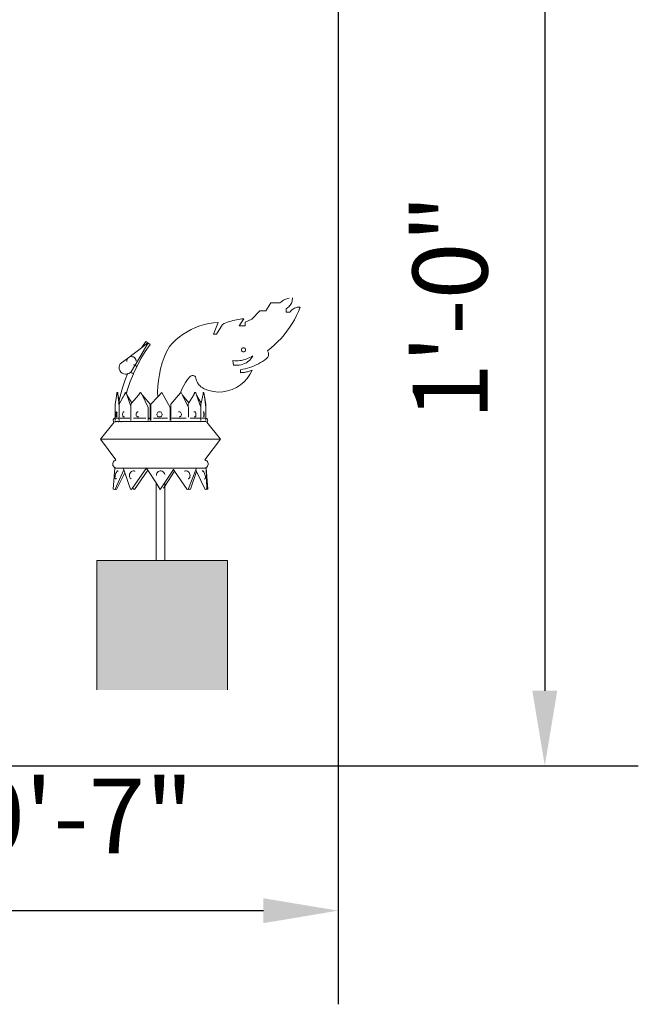
# Model space of a CAD drawing. Units: millimetres. Extents: x 7894 to 8038, y 6851 to 6951.
# Tile 27 of 49: x 7966.96 to 7975.23, y 6903.29 to 6916.43. Entities that reach past the tile are written whole.
import ezdxf

# ---------------------------------------------------------------- set-up
doc = ezdxf.new("R2010")
doc.units = ezdxf.units.MM
doc.layers.add('A-ANNO-DIMS', color=2, linetype='Continuous', lineweight=18)
doc.layers.add('A-FURN-ACCS', color=8, linetype='Continuous', lineweight=13)
doc.layers.add('A-FURN-ACCS-PATT', color=116, linetype='Continuous', lineweight=9, true_color=0x136734)
doc.styles.get("Standard").update_dxf_attribs({"font": 'arial.ttf'})
doc.dimstyles.new('ISO-25', dxfattribs={"dimtxt": 1, "dimasz": 1, "dimexe": 1.25, "dimexo": 0.625, "dimtad": 1, "dimdec": 0, "dimlunit": 4, "dimtxsty": 'Standard', "dimcen": 2.5, "dimclrt": 1, "dimadec": 0, "dimazin": 0, "dimtfac": 1, "dimtdec": 0, "dimtmove": 0, "dimatfit": 3, "dimfxl": 1, "dimarcsym": 0})

# ---------------------------------------------------------------- blocks, each defined once
blk = doc.blocks.new('DISPLAY-LEAF-FINIAL')
for p, q in [((2.209, 3.334), (2.276, 3.441)), ((2.276, 3.441), (2.398, 3.441)), ((2.398, 3.441), (2.409, 3.452)), ((2.409, 3.452), (2.421, 3.461)), ((2.421, 3.461), (2.434, 3.47)), ((2.434, 3.47), (2.447, 3.478)), ((2.447, 3.478), (2.461, 3.485)), ((2.461, 3.485), (2.475, 3.491)), ((2.475, 3.491), (2.489, 3.496)), ((2.489, 3.496), (2.504, 3.501)), ((2.504, 3.501), (2.519, 3.504)), ((2.544, 3.424), (2.536, 3.411)), ((2.551, 3.437), (2.544, 3.424)), ((2.556, 3.45), (2.551, 3.437)), ((2.56, 3.465), (2.556, 3.45)), ((2.563, 3.479), (2.56, 3.465)), ((2.565, 3.494), (2.563, 3.479)), ((2.565, 3.508), (2.565, 3.494)), ((2.023, 3.221), (2.127, 3.334)), ((2.127, 3.334), (2.209, 3.334)), ((2.493, 3.371), (2.48, 3.364)), ((2.48, 3.364), (2.48, 3.316)), ((2.48, 3.316), (2.533, 3.316)), ((2.505, 3.379), (2.493, 3.371)), ((2.516, 3.389), (2.505, 3.379)), ((2.527, 3.4), (2.516, 3.389)), ((2.536, 3.411), (2.527, 3.4)), ((2.533, 3.316), (2.54, 3.327)), ((2.54, 3.327), (2.549, 3.338)), ((2.549, 3.338), (2.558, 3.347)), ((2.558, 3.347), (2.569, 3.356)), ((2.569, 3.356), (2.58, 3.363)), ((2.58, 3.363), (2.592, 3.37)), ((2.592, 3.37), (2.604, 3.375)), ((2.604, 3.375), (2.617, 3.379)), ((2.617, 3.379), (2.63, 3.382)), ((2.646, 3.325), (2.62, 3.27)), ((2.63, 3.382), (2.643, 3.383)), ((2.643, 3.383), (2.657, 3.383)), ((2.67, 3.382), (2.646, 3.325)), ((2.657, 3.383), (2.67, 3.382)), ((1.388, 3.15), (1.449, 3.164)), ((1.449, 3.164), (1.51, 3.173)), ((1.51, 3.173), (1.572, 3.179)), ((1.572, 3.179), (1.511, 3.024)), ((1.632, 3.152), (1.654, 3.163)), ((1.654, 3.163), (1.676, 3.173)), ((1.676, 3.173), (1.699, 3.182)), ((1.699, 3.182), (1.722, 3.191)), ((1.722, 3.191), (1.745, 3.198)), ((1.745, 3.198), (1.769, 3.205)), ((1.769, 3.205), (1.793, 3.211)), ((1.793, 3.211), (1.817, 3.216)), ((1.817, 3.216), (1.841, 3.22)), ((1.841, 3.22), (1.865, 3.223)), ((1.914, 3.227), (1.854, 3.133)), ((1.865, 3.223), (1.889, 3.226)), ((1.889, 3.226), (1.914, 3.227)), ((1.934, 3.185), (2.023, 3.221)), ((1.934, 3.133), (1.934, 3.185)), ((2.56, 3.163), (2.527, 3.112)), ((2.591, 3.216), (2.56, 3.163)), ((2.62, 3.27), (2.591, 3.216)), ((1.105, 3.023), (1.158, 3.056)), ((1.158, 3.056), (1.213, 3.085)), ((1.213, 3.085), (1.27, 3.111)), ((1.27, 3.111), (1.328, 3.133)), ((1.328, 3.133), (1.388, 3.15)), ((1.511, 3.024), (1.55, 3.024)), ((1.55, 3.024), (1.632, 3.152)), ((1.854, 3.133), (1.934, 3.133)), ((2.491, 3.062), (2.453, 3.014)), ((2.527, 3.112), (2.491, 3.062)), ((0.634, 2.9), (0.463, 2.609)), ((0.605, 2.924), (0.547, 2.84)), ((0.634, 2.905), (0.547, 2.84)), ((0.634, 2.905), (0.605, 2.924)), ((0.634, 2.9), (0.634, 2.905)), ((0.663, 2.885), (0.634, 2.905)), ((0.92, 2.857), (0.962, 2.903)), ((0.962, 2.903), (1.007, 2.946)), ((1.007, 2.946), (1.055, 2.986)), ((1.055, 2.986), (1.105, 3.023)), ((2.371, 2.923), (2.327, 2.88)), ((2.413, 2.967), (2.371, 2.923)), ((2.453, 3.014), (2.413, 2.967)), ((0.547, 2.84), (0.379, 2.713)), ((0.541, 2.696), (0.599, 2.791)), ((0.599, 2.791), (0.663, 2.885)), ((0.884, 2.786), (0.853, 2.713)), ((0.92, 2.857), (0.884, 2.786)), ((1.883, 2.817), (1.885, 2.824)), ((1.883, 2.81), (1.883, 2.817)), ((1.885, 2.803), (1.883, 2.81)), ((1.885, 2.824), (1.889, 2.831)), ((1.888, 2.797), (1.885, 2.803)), ((1.894, 2.791), (1.888, 2.797)), ((1.889, 2.831), (1.894, 2.836)), ((1.894, 2.836), (1.9, 2.839)), ((1.9, 2.788), (1.894, 2.791)), ((1.9, 2.839), (1.907, 2.841)), ((1.907, 2.786), (1.9, 2.788)), ((1.907, 2.841), (1.914, 2.841)), ((1.914, 2.786), (1.907, 2.786)), ((1.914, 2.841), (1.921, 2.839)), ((1.921, 2.788), (1.914, 2.786)), ((1.921, 2.839), (1.928, 2.836)), ((1.928, 2.791), (1.921, 2.788)), ((1.928, 2.836), (1.933, 2.83)), ((1.933, 2.796), (1.928, 2.791)), ((1.933, 2.83), (1.937, 2.824)), ((1.936, 2.803), (1.933, 2.796)), ((1.938, 2.81), (1.936, 2.803)), ((1.937, 2.824), (1.938, 2.817)), ((1.938, 2.817), (1.938, 2.81)), ((2.281, 2.839), (2.233, 2.801)), ((2.233, 2.801), (2.238, 2.792)), ((2.238, 2.792), (2.242, 2.783)), ((2.242, 2.783), (2.245, 2.774)), ((2.245, 2.774), (2.246, 2.764)), ((2.246, 2.764), (2.246, 2.754)), ((2.327, 2.88), (2.281, 2.839)), ((0.379, 2.713), (0.264, 2.627)), ((0.353, 2.675), (0.358, 2.69)), ((0.353, 2.66), (0.353, 2.675)), ((0.353, 2.659), (0.353, 2.66)), ((0.353, 2.657), (0.353, 2.659)), ((0.358, 2.69), (0.367, 2.703)), ((0.367, 2.703), (0.379, 2.713)), ((0.379, 2.713), (0.393, 2.72)), ((0.393, 2.72), (0.409, 2.723)), ((0.409, 2.723), (0.425, 2.722)), ((0.425, 2.722), (0.44, 2.718)), ((0.44, 2.718), (0.453, 2.709)), ((0.453, 2.709), (0.464, 2.698)), ((0.464, 2.698), (0.471, 2.684)), ((0.471, 2.684), (0.475, 2.669)), ((0.474, 2.667), (0.475, 2.669)), ((0.474, 2.667), (0.475, 2.666)), ((0.541, 2.696), (0.488, 2.597)), ((0.826, 2.638), (0.804, 2.562)), ((0.853, 2.713), (0.826, 2.638)), ((1.793, 2.668), (1.77, 2.67)), ((1.77, 2.67), (1.776, 2.611)), ((1.816, 2.667), (1.793, 2.668)), ((1.84, 2.668), (1.816, 2.667)), ((1.863, 2.67), (1.84, 2.668)), ((1.886, 2.673), (1.863, 2.67)), ((1.909, 2.678), (1.886, 2.673)), ((1.926, 2.63), (1.902, 2.62)), ((1.931, 2.684), (1.909, 2.678)), ((1.949, 2.642), (1.926, 2.63)), ((1.954, 2.692), (1.931, 2.684)), ((1.97, 2.657), (1.949, 2.642)), ((1.975, 2.701), (1.954, 2.692)), ((1.99, 2.673), (1.97, 2.657)), ((1.996, 2.711), (1.975, 2.701)), ((2.007, 2.692), (1.99, 2.673)), ((2.017, 2.722), (1.996, 2.711)), ((2.023, 2.712), (2.007, 2.692)), ((2.036, 2.734), (2.017, 2.722)), ((2.036, 2.734), (2.023, 2.712)), ((2.137, 2.643), (2.11, 2.627)), ((2.164, 2.659), (2.137, 2.643)), ((2.19, 2.677), (2.164, 2.659)), ((2.216, 2.695), (2.19, 2.677)), ((2.223, 2.702), (2.216, 2.695)), ((2.23, 2.709), (2.223, 2.702)), ((2.235, 2.717), (2.23, 2.709)), ((2.24, 2.726), (2.235, 2.717)), ((2.243, 2.735), (2.24, 2.726)), ((2.245, 2.745), (2.243, 2.735)), ((2.246, 2.754), (2.245, 2.745)), ((0.253, 2.607), (0.249, 2.584)), ((0.249, 2.58), (0.249, 2.584)), ((0.249, 2.58), (0.251, 2.557)), ((0.251, 2.557), (0.259, 2.536)), ((0.264, 2.627), (0.253, 2.607)), ((0.259, 2.536), (0.272, 2.517)), ((0.272, 2.517), (0.29, 2.502)), ((0.29, 2.502), (0.311, 2.492)), ((0.38, 2.497), (0.4, 2.51)), ((0.398, 2.513), (0.402, 2.512)), ((0.403, 2.513), (0.4, 2.514)), ((0.4, 2.51), (0.402, 2.512)), ((0.402, 2.512), (0.403, 2.513)), ((0.402, 2.512), (0.44, 2.495)), ((0.403, 2.513), (0.415, 2.527)), ((0.403, 2.513), (0.44, 2.496)), ((0.409, 2.511), (0.408, 2.509)), ((0.42, 2.535), (0.409, 2.511)), ((0.414, 2.606), (0.413, 2.603)), ((0.461, 2.605), (0.415, 2.527)), ((0.44, 2.496), (0.486, 2.593)), ((0.443, 2.613), (0.446, 2.612)), ((0.451, 2.615), (0.449, 2.616)), ((0.463, 2.609), (0.461, 2.605)), ((0.486, 2.593), (0.461, 2.605)), ((0.463, 2.609), (0.488, 2.597)), ((0.804, 2.562), (0.787, 2.485)), ((1.801, 2.608), (1.776, 2.611)), ((1.827, 2.607), (1.801, 2.608)), ((1.852, 2.609), (1.827, 2.607)), ((1.878, 2.613), (1.852, 2.609)), ((1.903, 2.554), (1.872, 2.548)), ((1.872, 2.548), (1.872, 2.508)), ((1.872, 2.508), (1.885, 2.509)), ((1.902, 2.62), (1.878, 2.613)), ((1.885, 2.509), (1.898, 2.51)), ((1.898, 2.51), (1.911, 2.511)), ((1.934, 2.561), (1.903, 2.554)), ((1.911, 2.511), (1.924, 2.513)), ((1.924, 2.513), (1.937, 2.515)), ((1.964, 2.569), (1.934, 2.561)), ((1.937, 2.515), (1.95, 2.518)), ((1.95, 2.518), (1.963, 2.521)), ((1.963, 2.521), (1.976, 2.524)), ((1.994, 2.578), (1.964, 2.569)), ((1.976, 2.524), (1.988, 2.528)), ((1.988, 2.528), (2.001, 2.532)), ((2.024, 2.588), (1.994, 2.578)), ((2.026, 2.541), (1.997, 2.484)), ((2.001, 2.532), (2.013, 2.536)), ((2.013, 2.536), (2.026, 2.541)), ((2.053, 2.6), (2.024, 2.588)), ((2.082, 2.613), (2.053, 2.6)), ((2.11, 2.627), (2.082, 2.613)), ((0.332, 2.415), (0.295, 2.306)), ((0.311, 2.492), (0.334, 2.488)), ((0.363, 2.491), (0.332, 2.415)), ((0.334, 2.488), (0.358, 2.489)), ((0.358, 2.489), (0.363, 2.491)), ((0.361, 2.285), (0.398, 2.391)), ((0.363, 2.491), (0.38, 2.497)), ((0.365, 2.496), (0.363, 2.491)), ((0.398, 2.391), (0.44, 2.495)), ((0.774, 2.406), (0.766, 2.327)), ((0.787, 2.485), (0.774, 2.406)), ((1.136, 2.379), (1.113, 2.339)), ((1.163, 2.417), (1.136, 2.379)), ((1.193, 2.452), (1.163, 2.417)), ((1.198, 2.457), (1.193, 2.452)), ((1.204, 2.462), (1.198, 2.457)), ((1.211, 2.465), (1.204, 2.462)), ((1.218, 2.467), (1.211, 2.465)), ((1.225, 2.469), (1.218, 2.467)), ((1.232, 2.47), (1.225, 2.469)), ((1.239, 2.469), (1.232, 2.47)), ((1.247, 2.467), (1.239, 2.469)), ((1.254, 2.465), (1.247, 2.467)), ((1.26, 2.462), (1.254, 2.465)), ((1.266, 2.457), (1.26, 2.462)), ((1.271, 2.452), (1.266, 2.457)), ((1.274, 2.435), (1.271, 2.452)), ((1.278, 2.418), (1.274, 2.435)), ((1.283, 2.402), (1.278, 2.418)), ((1.29, 2.386), (1.283, 2.402)), ((1.298, 2.371), (1.29, 2.386)), ((1.308, 2.357), (1.298, 2.371)), ((1.918, 2.385), (1.87, 2.344)), ((1.961, 2.432), (1.918, 2.385)), ((1.997, 2.484), (1.961, 2.432)), ((0.215, 2.201), (0.22, 2.245)), ((0.223, 2.245), (0.215, 2.201)), ((0.223, 2.245), (0.22, 2.245)), ((0.223, 2.245), (0.23, 2.245)), ((0.232, 2.22), (0.23, 2.245)), ((0.295, 2.306), (0.263, 2.194)), ((0.317, 2.207), (0.33, 2.245)), ((0.338, 2.245), (0.317, 2.207)), ((0.332, 2.245), (0.33, 2.245)), ((0.344, 2.245), (0.338, 2.245)), ((0.347, 2.235), (0.344, 2.245)), ((0.347, 2.235), (0.361, 2.285)), ((0.507, 2.209), (0.525, 2.245)), ((0.532, 2.239), (0.507, 2.209)), ((0.528, 2.245), (0.525, 2.245)), ((0.528, 2.245), (0.532, 2.239)), ((0.537, 2.245), (0.532, 2.239)), ((0.54, 2.245), (0.537, 2.245)), ((0.556, 2.211), (0.54, 2.245)), ((0.766, 2.327), (0.763, 2.248)), ((0.763, 2.248), (0.765, 2.186)), ((0.821, 2.245), (0.765, 2.186)), ((0.93, 2.045), (0.821, 2.245)), ((1.07, 2.239), (0.939, 2.086)), ((1.07, 2.239), (1.069, 2.235)), ((1.071, 2.24), (1.07, 2.239)), ((1.07, 2.239), (1.071, 2.237)), ((1.075, 2.254), (1.071, 2.24)), ((1.074, 2.245), (1.071, 2.24)), ((1.074, 2.245), (1.078, 2.245)), ((1.092, 2.297), (1.075, 2.254)), ((1.095, 2.209), (1.078, 2.245)), ((1.113, 2.339), (1.092, 2.297)), ((1.248, 2.213), (1.258, 2.245)), ((1.265, 2.242), (1.248, 2.213)), ((1.258, 2.245), (1.264, 2.245)), ((1.264, 2.245), (1.265, 2.242)), ((1.267, 2.245), (1.265, 2.242)), ((1.267, 2.245), (1.272, 2.245)), ((1.285, 2.207), (1.272, 2.245)), ((1.319, 2.343), (1.308, 2.357)), ((1.331, 2.331), (1.319, 2.343)), ((1.343, 2.319), (1.331, 2.331)), ((1.357, 2.309), (1.343, 2.319)), ((1.372, 2.3), (1.357, 2.309)), ((1.37, 2.22), (1.372, 2.245)), ((1.375, 2.245), (1.37, 2.22)), ((1.387, 2.292), (1.372, 2.3)), ((1.372, 2.245), (1.375, 2.245)), ((1.375, 2.245), (1.382, 2.245)), ((1.382, 2.245), (1.389, 2.19)), ((1.447, 2.27), (1.387, 2.292)), ((1.509, 2.256), (1.447, 2.27)), ((1.572, 2.25), (1.509, 2.256)), ((1.635, 2.253), (1.572, 2.25)), ((1.698, 2.264), (1.635, 2.253)), ((1.759, 2.283), (1.698, 2.264)), ((1.816, 2.31), (1.759, 2.283)), ((1.87, 2.344), (1.816, 2.31)), ((0.213, 2.19), (0.195, 2.086)), ((0.213, 2.19), (0.215, 2.201)), ((0.232, 2.22), (0.25, 2.138)), ((0.244, 2.11), (0.232, 2.22)), ((0.244, 2.11), (0.239, 2.089)), ((0.25, 2.138), (0.244, 2.11)), ((0.248, 2.065), (0.244, 2.11)), ((0.317, 2.207), (0.248, 2.086)), ((0.263, 2.194), (0.25, 2.138)), ((0.25, 2.138), (0.256, 2.115)), ((0.297, 2.185), (0.292, 2.162)), ((0.354, 2.213), (0.347, 2.235)), ((0.354, 2.213), (0.42, 2.104)), ((0.404, 2.061), (0.354, 2.213)), ((0.42, 2.104), (0.404, 2.086)), ((0.507, 2.209), (0.42, 2.104)), ((0.548, 2.22), (0.556, 2.211)), ((0.556, 2.211), (0.663, 2.086)), ((0.636, 2.045), (0.556, 2.211)), ((0.765, 2.186), (0.671, 2.086)), ((1.095, 2.209), (1.182, 2.104)), ((1.095, 2.209), (1.171, 2.054)), ((1.182, 2.104), (1.171, 2.086)), ((1.248, 2.213), (1.182, 2.104)), ((1.285, 2.207), (1.344, 2.103)), ((1.285, 2.207), (1.34, 2.048)), ((1.37, 2.22), (1.344, 2.103)), ((1.389, 2.19), (1.408, 2.086)), ((1.407, 2.045), (1.389, 2.19)), ((0.195, 2.086), (0.195, 2.048)), ((0.195, 2.045), (0.195, 2.048)), ((0.195, 2.045), (0.195, 1.903)), ((0.207, 1.965), (0.208, 1.973)), ((0.208, 1.973), (0.209, 1.979)), ((0.209, 1.979), (0.211, 1.984)), ((0.211, 1.984), (0.213, 1.986)), ((0.211, 1.965), (0.212, 1.973)), ((0.212, 1.973), (0.213, 1.979)), ((0.216, 1.986), (0.213, 1.986)), ((0.213, 1.979), (0.214, 1.984)), ((0.214, 1.984), (0.216, 1.986)), ((0.218, 1.973), (0.217, 1.965)), ((0.219, 1.979), (0.218, 1.973)), ((0.218, 1.973), (0.218, 1.967)), ((0.22, 1.981), (0.219, 1.979)), ((0.22, 1.981), (0.219, 1.979)), ((0.221, 1.973), (0.22, 1.965)), ((0.222, 1.975), (0.221, 1.973)), ((0.248, 2.086), (0.248, 2.065)), ((0.248, 2.065), (0.248, 1.903)), ((0.297, 1.965), (0.3, 1.973)), ((0.3, 1.973), (0.304, 1.979)), ((0.304, 1.979), (0.308, 1.984)), ((0.308, 1.984), (0.314, 1.986)), ((0.316, 1.986), (0.314, 1.986)), ((0.404, 2.086), (0.404, 2.061)), ((0.404, 2.061), (0.404, 1.901)), ((0.478, 1.965), (0.482, 1.973)), ((0.482, 1.973), (0.488, 1.979)), ((0.488, 1.979), (0.495, 1.984)), ((0.495, 1.984), (0.502, 1.986)), ((0.504, 1.986), (0.502, 1.986)), ((0.636, 2.045), (0.637, 1.903)), ((0.663, 2.086), (0.663, 1.903)), ((0.671, 2.086), (0.671, 1.903)), ((0.756, 1.965), (0.761, 1.973)), ((0.761, 1.973), (0.767, 1.979)), ((0.767, 1.979), (0.775, 1.984)), ((0.775, 1.984), (0.784, 1.986)), ((0.784, 1.986), (0.793, 1.986)), ((0.793, 1.986), (0.802, 1.984)), ((0.802, 1.984), (0.81, 1.979)), ((0.81, 1.979), (0.816, 1.973)), ((0.816, 1.973), (0.821, 1.965)), ((0.93, 2.045), (0.931, 1.934)), ((0.939, 2.086), (0.939, 1.934)), ((1.044, 1.986), (1.046, 1.986)), ((1.046, 1.986), (1.054, 1.986)), ((1.054, 1.986), (1.062, 1.984)), ((1.062, 1.984), (1.069, 1.979)), ((1.069, 1.979), (1.075, 1.973)), ((1.075, 1.973), (1.079, 1.965)), ((1.171, 2.086), (1.171, 2.054)), ((1.176, 2.045), (1.171, 2.054)), ((1.176, 2.045), (1.177, 1.914)), ((1.249, 1.986), (1.251, 1.986)), ((1.251, 1.986), (1.257, 1.986)), ((1.257, 1.986), (1.263, 1.984)), ((1.263, 1.984), (1.268, 1.979)), ((1.268, 1.979), (1.272, 1.973)), ((1.272, 1.973), (1.275, 1.965)), ((1.344, 2.103), (1.34, 2.086)), ((1.34, 2.086), (1.34, 2.048)), ((1.341, 2.045), (1.34, 2.048)), ((1.341, 2.045), (1.342, 1.903)), ((1.373, 1.986), (1.376, 1.986)), ((1.376, 1.986), (1.378, 1.984)), ((1.376, 1.986), (1.377, 1.986)), ((1.377, 1.986), (1.379, 1.986)), ((1.378, 1.984), (1.379, 1.979)), ((1.379, 1.986), (1.381, 1.984)), ((1.379, 1.979), (1.381, 1.973)), ((1.381, 1.984), (1.383, 1.979)), ((1.381, 1.973), (1.382, 1.965)), ((1.383, 1.979), (1.384, 1.973)), ((1.384, 1.973), (1.385, 1.965)), ((1.408, 2.086), (1.407, 2.045)), ((1.407, 2.045), (1.408, 1.903)), ((0, 1.62), (0.181, 1.849)), ((0.17, 1.877), (0.172, 1.885)), ((0.17, 1.87), (0.17, 1.877)), ((0.172, 1.862), (0.17, 1.87)), ((0.172, 1.885), (0.176, 1.892)), ((0.175, 1.855), (0.172, 1.862)), ((0.181, 1.849), (0.175, 1.855)), ((0.176, 1.892), (0.182, 1.898)), ((0.182, 1.898), (0.189, 1.901)), ((0.189, 1.901), (0.195, 1.903)), ((0.195, 1.903), (0.195, 1.901)), ((0.195, 1.903), (0.196, 1.903)), ((0.195, 1.898), (0.195, 1.87)), ((0.195, 1.862), (0.195, 1.855)), ((0.195, 1.855), (0.195, 1.855)), ((0.205, 1.855), (0.195, 1.855)), ((0.196, 1.903), (0.198, 1.903)), ((0.196, 1.903), (0.197, 1.903)), ((0.237, 1.903), (0.198, 1.903)), ((0.205, 1.855), (0.205, 1.851)), ((0.248, 1.855), (0.205, 1.855)), ((0.205, 1.851), (0.205, 1.849)), ((0.207, 1.956), (0.207, 1.965)), ((0.207, 1.947), (0.207, 1.956)), ((0.207, 1.938), (0.207, 1.947)), ((0.208, 1.93), (0.207, 1.938)), ((0.209, 1.924), (0.208, 1.93)), ((0.211, 1.919), (0.209, 1.924)), ((0.21, 1.956), (0.211, 1.965)), ((0.21, 1.947), (0.21, 1.956)), ((0.211, 1.938), (0.21, 1.947)), ((0.212, 1.93), (0.211, 1.938)), ((0.213, 1.917), (0.211, 1.919)), ((0.213, 1.924), (0.212, 1.93)), ((0.216, 1.947), (0.213, 1.924)), ((0.214, 1.919), (0.213, 1.924)), ((0.214, 1.917), (0.213, 1.917)), ((0.216, 1.917), (0.214, 1.919)), ((0.216, 1.917), (0.214, 1.917)), ((0.217, 1.965), (0.216, 1.956)), ((0.216, 1.956), (0.216, 1.947)), ((0.216, 1.947), (0.217, 1.938)), ((0.218, 1.917), (0.216, 1.917)), ((0.218, 1.967), (0.217, 1.965)), ((0.217, 1.938), (0.218, 1.93)), ((0.218, 1.93), (0.219, 1.924)), ((0.219, 1.924), (0.22, 1.921)), ((0.22, 1.965), (0.22, 1.956)), ((0.22, 1.956), (0.22, 1.947)), ((0.22, 1.947), (0.22, 1.938)), ((0.22, 1.938), (0.221, 1.93)), ((0.221, 1.93), (0.222, 1.928)), ((0.24, 1.855), (0.24, 1.849)), ((0.248, 1.903), (0.244, 1.903)), ((0.245, 1.898), (0.244, 1.886)), ((0.248, 1.897), (0.244, 1.897)), ((0.248, 1.925), (0.246, 1.901)), ((0.248, 1.903), (0.248, 1.901)), ((0.248, 1.898), (0.248, 1.897)), ((0.248, 1.897), (0.248, 1.87)), ((0.248, 1.862), (0.248, 1.855)), ((0.248, 1.855), (0.276, 1.855)), ((0.391, 1.903), (0.265, 1.903)), ((0.275, 1.849), (0.276, 1.855)), ((0.276, 1.855), (0.405, 1.855)), ((0.295, 1.956), (0.297, 1.965)), ((0.295, 1.947), (0.295, 1.956)), ((0.297, 1.938), (0.295, 1.947)), ((0.3, 1.93), (0.297, 1.938)), ((0.303, 1.924), (0.3, 1.93)), ((0.308, 1.919), (0.303, 1.924)), ((0.313, 1.917), (0.308, 1.919)), ((0.319, 1.917), (0.313, 1.917)), ((0.322, 1.917), (0.319, 1.917)), ((0.404, 1.898), (0.404, 1.87)), ((0.404, 1.862), (0.405, 1.855)), ((0.405, 1.855), (0.637, 1.855)), ((0.439, 1.903), (0.607, 1.903)), ((0.476, 1.956), (0.478, 1.965)), ((0.476, 1.947), (0.476, 1.956)), ((0.478, 1.938), (0.476, 1.947)), ((0.482, 1.93), (0.478, 1.938)), ((0.488, 1.924), (0.482, 1.93)), ((0.495, 1.919), (0.488, 1.924)), ((0.502, 1.917), (0.495, 1.919)), ((0.51, 1.917), (0.502, 1.917)), ((0.512, 1.917), (0.51, 1.917)), ((0.637, 1.903), (0.634, 1.903)), ((0.637, 1.897), (0.634, 1.897)), ((0.637, 1.903), (0.637, 1.901)), ((0.663, 1.903), (0.637, 1.903)), ((0.637, 1.898), (0.637, 1.897)), ((0.637, 1.897), (0.637, 1.87)), ((0.663, 1.897), (0.637, 1.897)), ((0.637, 1.862), (0.637, 1.855)), ((0.663, 1.855), (0.637, 1.855)), ((0.663, 1.903), (0.671, 1.903)), ((0.663, 1.903), (0.663, 1.901)), ((0.663, 1.898), (0.663, 1.897)), ((0.663, 1.897), (0.663, 1.87)), ((0.671, 1.897), (0.663, 1.897)), ((0.663, 1.862), (0.663, 1.855)), ((0.671, 1.903), (0.671, 1.901)), ((0.671, 1.898), (0.671, 1.897)), ((0.671, 1.897), (0.671, 1.87)), ((0.671, 1.862), (0.671, 1.855)), ((0.671, 1.855), (0.932, 1.855)), ((0.708, 1.903), (0.894, 1.903)), ((0.754, 1.956), (0.756, 1.965)), ((0.754, 1.947), (0.754, 1.956)), ((0.756, 1.938), (0.754, 1.947)), ((0.761, 1.93), (0.756, 1.938)), ((0.767, 1.924), (0.761, 1.93)), ((0.775, 1.919), (0.767, 1.924)), ((0.784, 1.917), (0.775, 1.919)), ((0.793, 1.917), (0.784, 1.917)), ((0.802, 1.919), (0.793, 1.917)), ((0.81, 1.924), (0.802, 1.919)), ((0.816, 1.93), (0.81, 1.924)), ((0.821, 1.938), (0.816, 1.93)), ((0.821, 1.965), (0.823, 1.956)), ((0.823, 1.947), (0.821, 1.938)), ((0.823, 1.956), (0.823, 1.947)), ((0.939, 1.934), (0.931, 1.934)), ((0.931, 1.934), (0.931, 1.903)), ((0.931, 1.903), (0.931, 1.901)), ((0.939, 1.903), (0.931, 1.903)), ((0.931, 1.898), (0.931, 1.897)), ((0.931, 1.897), (0.932, 1.87)), ((0.939, 1.897), (0.931, 1.897)), ((0.932, 1.862), (0.932, 1.855)), ((0.939, 1.855), (0.932, 1.855)), ((0.942, 1.934), (0.939, 1.934)), ((0.939, 1.934), (0.939, 1.903)), ((0.942, 1.903), (0.939, 1.903)), ((0.939, 1.903), (0.939, 1.901)), ((0.939, 1.898), (0.939, 1.897)), ((0.942, 1.897), (0.939, 1.897)), ((0.939, 1.897), (0.939, 1.87)), ((0.939, 1.862), (0.939, 1.855)), ((1.342, 1.855), (0.939, 1.855)), ((0.953, 1.903), (1.146, 1.903)), ((1.022, 1.935), (1.021, 1.935)), ((1.052, 1.917), (1.054, 1.917)), ((1.062, 1.919), (1.054, 1.917)), ((1.069, 1.924), (1.062, 1.919)), ((1.075, 1.93), (1.069, 1.924)), ((1.079, 1.938), (1.075, 1.93)), ((1.079, 1.965), (1.081, 1.956)), ((1.081, 1.947), (1.079, 1.938)), ((1.081, 1.956), (1.081, 1.947)), ((1.33, 1.903), (1.197, 1.903)), ((1.254, 1.917), (1.257, 1.917)), ((1.263, 1.919), (1.257, 1.917)), ((1.268, 1.924), (1.263, 1.919)), ((1.272, 1.93), (1.268, 1.924)), ((1.275, 1.938), (1.272, 1.93)), ((1.275, 1.965), (1.276, 1.956)), ((1.276, 1.947), (1.275, 1.938)), ((1.276, 1.956), (1.276, 1.947)), ((1.347, 1.903), (1.342, 1.903)), ((1.342, 1.903), (1.342, 1.901)), ((1.342, 1.898), (1.342, 1.897)), ((1.347, 1.897), (1.342, 1.897)), ((1.342, 1.897), (1.342, 1.87)), ((1.342, 1.862), (1.342, 1.855)), ((1.408, 1.855), (1.342, 1.855)), ((1.356, 1.903), (1.4, 1.903)), ((1.378, 1.919), (1.375, 1.917)), ((1.375, 1.917), (1.379, 1.917)), ((1.379, 1.924), (1.378, 1.919)), ((1.381, 1.93), (1.379, 1.924)), ((1.381, 1.919), (1.379, 1.917)), ((1.382, 1.938), (1.381, 1.93)), ((1.383, 1.924), (1.381, 1.919)), ((1.382, 1.965), (1.382, 1.956)), ((1.382, 1.956), (1.382, 1.947)), ((1.382, 1.947), (1.382, 1.938)), ((1.384, 1.93), (1.383, 1.924)), ((1.385, 1.938), (1.384, 1.93)), ((1.385, 1.965), (1.386, 1.956)), ((1.386, 1.947), (1.385, 1.938)), ((1.386, 1.956), (1.386, 1.947)), ((1.408, 1.903), (1.413, 1.901)), ((1.408, 1.903), (1.408, 1.901)), ((1.408, 1.898), (1.408, 1.87)), ((1.408, 1.862), (1.408, 1.855)), ((1.413, 1.901), (1.42, 1.898)), ((1.42, 1.898), (1.426, 1.892)), ((1.427, 1.855), (1.421, 1.849)), ((1.421, 1.849), (1.602, 1.62)), ((1.426, 1.892), (1.43, 1.885)), ((1.431, 1.862), (1.427, 1.855)), ((1.43, 1.885), (1.432, 1.877)), ((1.433, 1.87), (1.431, 1.862)), ((1.432, 1.877), (1.433, 1.87)), ((0.207, 1.343), (0, 1.62)), ((1.602, 1.62), (0, 1.62)), ((1.602, 1.62), (1.395, 1.343)), ((0.168, 1.31), (0.174, 1.321)), ((0.174, 1.321), (0.183, 1.331)), ((0.183, 1.331), (0.195, 1.338)), ((0.195, 1.338), (0.207, 1.343)), ((1.395, 1.343), (1.408, 1.338)), ((1.408, 1.338), (1.419, 1.331)), ((1.419, 1.331), (1.428, 1.321)), ((1.428, 1.321), (1.434, 1.31)), ((0.164, 1.297), (0.168, 1.31)), ((0.164, 1.283), (0.164, 1.297)), ((0.167, 1.27), (0.164, 1.283)), ((0.173, 1.258), (0.167, 1.27)), ((0.171, 0.955), (0.191, 1.234)), ((0.182, 1.248), (0.173, 1.258)), ((0.193, 1.24), (0.182, 1.248)), ((0.219, 1.234), (0.191, 1.234)), ((0.206, 1.236), (0.193, 1.24)), ((0.196, 0.954), (0.311, 1.21)), ((0.219, 1.234), (0.206, 1.236)), ((0.212, 1.177), (0.217, 1.187)), ((0.217, 1.187), (0.223, 1.193)), ((0.219, 1.234), (0.297, 1.234)), ((0.223, 1.193), (0.228, 1.197)), ((0.228, 1.197), (0.232, 1.196)), ((0.232, 1.195), (0.232, 1.196)), ((0.232, 1.195), (0.237, 1.195)), ((0.297, 1.234), (0.302, 1.234)), ((0.303, 1.232), (0.297, 1.234)), ((0.303, 1.232), (0.302, 1.234)), ((0.302, 1.234), (0.594, 1.234)), ((0.311, 1.21), (0.303, 1.232)), ((0.324, 1.172), (0.311, 1.21)), ((0.403, 1.177), (0.413, 1.187)), ((0.413, 1.187), (0.424, 1.193)), ((0.424, 1.193), (0.436, 1.197)), ((0.434, 0.975), (0.609, 1.228)), ((0.436, 1.197), (0.448, 1.196)), ((0.448, 1.196), (0.458, 1.192)), ((0.455, 0.949), (0.632, 1.205)), ((0.458, 1.192), (0.461, 1.191)), ((0.594, 1.234), (0.617, 1.234)), ((0.609, 1.228), (0.594, 1.234)), ((0.617, 1.228), (0.617, 1.234)), ((0.952, 1.234), (0.617, 1.234)), ((0.632, 1.205), (0.617, 1.228)), ((0.742, 1.037), (0.632, 1.205)), ((0.76, 1.177), (0.77, 1.187)), ((0.77, 1.187), (0.783, 1.193)), ((0.783, 1.193), (0.797, 1.197)), ((0.797, 1.197), (0.812, 1.196)), ((0.812, 1.196), (0.826, 1.192)), ((0.826, 1.192), (0.838, 1.185)), ((0.838, 1.185), (0.848, 1.175)), ((0.86, 1.041), (0.977, 1.215)), ((0.86, 0.992), (0.99, 1.195)), ((0.981, 1.234), (0.952, 1.234)), ((0.977, 1.215), (0.974, 1.218)), ((0.99, 1.195), (0.977, 1.215)), ((0.981, 1.234), (0.982, 1.234)), ((0.982, 1.234), (0.983, 1.234)), ((1.284, 1.234), (0.983, 1.234)), ((1.16, 0.949), (0.99, 1.195)), ((1.124, 1.192), (1.126, 1.193)), ((1.126, 1.193), (1.127, 1.193)), ((1.127, 1.193), (1.138, 1.197)), ((1.138, 1.197), (1.15, 1.196)), ((1.15, 1.196), (1.162, 1.192)), ((1.162, 1.192), (1.174, 1.185)), ((1.174, 1.185), (1.184, 1.175)), ((1.177, 0.964), (1.275, 1.212)), ((1.202, 0.955), (1.285, 1.19)), ((1.275, 1.212), (1.283, 1.232)), ((1.285, 1.19), (1.275, 1.212)), ((1.283, 1.232), (1.29, 1.234)), ((1.283, 1.232), (1.284, 1.234)), ((1.284, 1.234), (1.29, 1.234)), ((1.398, 0.949), (1.285, 1.19)), ((1.29, 1.234), (1.383, 1.234)), ((1.359, 1.195), (1.364, 1.197)), ((1.359, 1.195), (1.362, 1.195)), ((1.364, 1.197), (1.369, 1.196)), ((1.369, 1.196), (1.374, 1.192)), ((1.374, 1.192), (1.38, 1.185)), ((1.38, 1.185), (1.386, 1.175)), ((1.397, 1.236), (1.383, 1.234)), ((1.41, 1.234), (1.383, 1.234)), ((1.409, 1.24), (1.397, 1.236)), ((1.42, 1.248), (1.409, 1.24)), ((1.411, 1.234), (1.41, 1.234)), ((1.411, 1.232), (1.411, 1.234)), ((1.435, 0.955), (1.411, 1.232)), ((1.42, 0.955), (1.411, 1.232)), ((1.429, 1.258), (1.42, 1.248)), ((1.435, 1.27), (1.429, 1.258)), ((1.434, 1.31), (1.438, 1.297)), ((1.438, 1.283), (1.435, 1.27)), ((1.438, 1.297), (1.438, 1.283)), ((0.194, 1.111), (0.196, 1.124)), ((0.195, 1.101), (0.194, 1.111)), ((0.196, 1.094), (0.195, 1.101)), ((0.196, 1.124), (0.198, 1.137)), ((0.199, 1.09), (0.196, 1.094)), ((0.198, 1.137), (0.202, 1.152)), ((0.203, 1.089), (0.199, 1.09)), ((0.202, 1.152), (0.206, 1.165)), ((0.204, 1.088), (0.203, 1.089)), ((0.206, 1.165), (0.212, 1.177)), ((0.211, 1.096), (0.213, 1.092)), ((0.213, 1.092), (0.214, 1.092)), ((0.214, 1.1), (0.214, 1.098)), ((0.215, 0.949), (0.324, 1.172)), ((0.402, 0.955), (0.324, 1.172)), ((0.387, 1.137), (0.389, 1.152)), ((0.387, 1.124), (0.387, 1.137)), ((0.391, 1.111), (0.387, 1.124)), ((0.389, 1.152), (0.395, 1.165)), ((0.397, 1.101), (0.391, 1.111)), ((0.395, 1.165), (0.403, 1.177)), ((0.406, 1.094), (0.397, 1.101)), ((0.409, 1.092), (0.406, 1.094)), ((0.747, 1.137), (0.748, 1.152)), ((0.747, 1.136), (0.747, 1.137)), ((0.748, 1.152), (0.752, 1.165)), ((0.752, 1.165), (0.76, 1.177)), ((0.848, 1.175), (0.855, 1.162)), ((0.855, 1.162), (0.859, 1.148)), ((0.859, 1.147), (0.859, 1.148)), ((1.174, 1.092), (1.172, 1.091)), ((1.174, 1.092), (1.175, 1.092)), ((1.185, 1.099), (1.175, 1.092)), ((1.184, 1.175), (1.191, 1.162)), ((1.192, 1.109), (1.185, 1.099)), ((1.191, 1.162), (1.196, 1.148)), ((1.196, 1.121), (1.192, 1.109)), ((1.196, 1.148), (1.198, 1.134)), ((1.198, 1.134), (1.196, 1.121)), ((1.386, 1.175), (1.392, 1.162)), ((1.392, 1.089), (1.39, 1.088)), ((1.39, 1.088), (1.395, 1.089)), ((1.392, 1.162), (1.396, 1.148)), ((1.399, 1.092), (1.395, 1.089)), ((1.396, 1.148), (1.4, 1.134)), ((1.401, 1.099), (1.399, 1.092)), ((1.4, 1.134), (1.402, 1.121)), ((1.402, 1.109), (1.401, 1.099)), ((1.402, 1.121), (1.402, 1.109)), ((0.194, 0.949), (0.171, 0.955)), ((0.194, 0.949), (0.196, 0.954)), ((0.215, 0.949), (0.196, 0.954)), ((0.416, 0.949), (0.402, 0.955)), ((0.416, 0.949), (0.434, 0.975)), ((0.442, 0.955), (0.434, 0.975)), ((0.455, 0.949), (0.442, 0.955)), ((0.742, 0), (0.742, 1.037)), ((0.799, 0.949), (0.742, 1.037)), ((0.799, 0.949), (0.816, 0.974)), ((0.816, 0.974), (0.814, 0.977)), ((0.816, 0.974), (0.86, 1.041)), ((0.816, 0.973), (0.816, 0.974)), ((0.843, 0.965), (0.86, 0.992)), ((0.86, 1.041), (0.86, 1.047)), ((0.86, 0.992), (0.86, 1.041)), ((0.86, 0), (0.86, 0.992)), ((1.16, 0.949), (1.173, 0.955)), ((1.173, 0.955), (1.177, 0.964)), ((1.187, 0.949), (1.177, 0.964)), ((1.187, 0.949), (1.202, 0.955)), ((1.398, 0.949), (1.41, 0.953)), ((1.41, 0.953), (1.42, 0.955)), ((1.412, 0.949), (1.41, 0.953)), ((1.412, 0.949), (1.435, 0.955))]:
    blk.add_line(p, q)
blk = doc.blocks.new('*D23')
at = {"layer": 'A-ANNO-DIMS', "color": 0, "lineweight": -2, "transparency": 16777216}
for p, q in [((7940.089, 6907.098), (7940.089, 6947.793)), ((7971.936, 6928.989), (7971.936, 6947.793)), ((7941.089, 6946.543), (7970.936, 6946.543))]:
    blk.add_line(p, q, dxfattribs=at)
at = {"layer": 'A-ANNO-DIMS', "color": 0, "transparency": 16777216}
for points in [[(7941.089, 6946.709), (7941.089, 6946.376), (7940.089, 6946.543)], [(7970.936, 6946.709), (7970.936, 6946.376), (7971.936, 6946.543)]]:
    blk.add_solid(points, dxfattribs=at)
at = {"layer": 'Defpoints', "color": 0, "transparency": 16777216}
for p in [(7971.936, 6946.543), (7971.936, 6928.364), (7940.089, 6906.473)]:
    blk.add_point(p, dxfattribs=at)
at = {"layer": 'A-ANNO-DIMS', "color": 1, "transparency": 16777216, "insert": (7956.012, 6947.678), "char_height": 1, "attachment_point": 5}
blk.add_mtext('2\'-8"', dxfattribs=at)
blk = doc.blocks.new('*D26')
at = {"layer": 'A-ANNO-DIMS', "color": 0, "lineweight": -2, "transparency": 16777216}
for p, q in [((7950.965, 6918.72), (7975.227, 6918.72)), ((7973.977, 6917.72), (7973.977, 6907.473)), ((7964.966, 6906.473), (7975.227, 6906.473))]:
    blk.add_line(p, q, dxfattribs=at)
at = {"layer": 'A-ANNO-DIMS', "color": 0, "transparency": 16777216}
for points in [[(7973.811, 6917.72), (7974.144, 6917.72), (7973.977, 6918.72)], [(7973.811, 6907.473), (7974.144, 6907.473), (7973.977, 6906.473)]]:
    blk.add_solid(points, dxfattribs=at)
at = {"layer": 'Defpoints', "color": 0, "transparency": 16777216}
for p in [(7950.34, 6918.72), (7964.341, 6906.473), (7973.977, 6906.473)]:
    blk.add_point(p, dxfattribs=at)
at = {"layer": 'A-ANNO-DIMS', "color": 1, "transparency": 16777216, "insert": (7972.842, 6912.597), "char_height": 1, "attachment_point": 5, "rotation": 90}
blk.add_mtext('1\'-0"', dxfattribs=at)
blk = doc.blocks.new('*D34')
at = {"layer": 'A-ANNO-DIMS', "color": 0, "lineweight": -2, "transparency": 16777216}
for p, q in [((7971.217, 6922.003), (7971.217, 6903.287)), ((7964.341, 6905.848), (7964.341, 6903.287)), ((7965.341, 6904.537), (7970.217, 6904.537))]:
    blk.add_line(p, q, dxfattribs=at)
at = {"layer": 'A-ANNO-DIMS', "color": 0, "transparency": 16777216}
for points in [[(7965.341, 6904.703), (7965.341, 6904.37), (7964.341, 6904.537)], [(7970.217, 6904.703), (7970.217, 6904.37), (7971.217, 6904.537)]]:
    blk.add_solid(points, dxfattribs=at)
at = {"layer": 'Defpoints', "color": 0, "transparency": 16777216}
for p in [(7971.217, 6922.628), (7964.341, 6906.473), (7971.217, 6904.537)]:
    blk.add_point(p, dxfattribs=at)
at = {"layer": 'A-ANNO-DIMS', "color": 1, "transparency": 16777216, "insert": (7967.779, 6905.672), "char_height": 1, "attachment_point": 5}
blk.add_mtext('0\'-7"', dxfattribs=at)

msp = doc.modelspace()

# ---------------------------------------------------------------- hatches: boundary and pattern name
at = {"layer": 'A-FURN-ACCS-PATT'}
h = msp.add_hatch(color=256, dxfattribs=at)
h.dxf.hatch_style = 1
h.paths.add_polyline_path([(7969.74, 6909.212), (7968.901, 6909.212), (7968.783, 6909.212), (7967.992, 6909.212), (7967.992, 6907.484), (7969.74, 6907.484)])

# ---------------------------------------------------------------- linework, layer by layer
at = {"layer": 'A-FURN-ACCS'}
for p, q in [((7967.992, 6907.484), (7967.992, 6909.212)), ((7967.992, 6909.212), (7968.783, 6909.212)), ((7968.901, 6909.212), (7968.783, 6909.212)), ((7968.901, 6909.212), (7969.74, 6909.212)), ((7969.74, 6907.484), (7969.74, 6909.212))]:
    msp.add_line(p, q, dxfattribs=at)

# ---------------------------------------------------------------- block references
msp.add_blockref('DISPLAY-LEAF-FINIAL', (7968.041, 6909.212), dxfattribs=at)

# ---------------------------------------------------------------- dimensions: what is measured, and where the dimension line sits
at = {"layer": 'A-ANNO-DIMS'}
for base, p1, p2, picture, middle in [((7971.936, 6946.543), (7940.089, 6906.473), (7971.936, 6928.364), '*D23', (7956.012, 6947.678)), ((7971.217, 6904.537), (7964.341, 6906.473), (7971.217, 6922.628), '*D34', (7967.779, 6905.672))]:
    dim = msp.add_linear_dim(base=base, p1=p1, p2=p2, dimstyle='ISO-25', override={"dimdec": 1, "dimlfac": 1, "dimrnd": 0, "dimzin": 1, "dimdsep": 46, "dimlunit": 4, "dimfrac": 2}, dxfattribs=at)
    dim.commit()
    dim.dimension.update_dxf_attribs({"geometry": picture, "text_midpoint": middle})
dim = msp.add_linear_dim(base=(7973.977, 6906.473), p1=(7950.34, 6918.72), p2=(7964.341, 6906.473), angle=90, dimstyle='ISO-25', override={"dimdec": 1, "dimlfac": 1, "dimrnd": 0, "dimzin": 1, "dimdsep": 46, "dimlunit": 4, "dimfrac": 2}, dxfattribs=at)
dim.commit()
dim.dimension.update_dxf_attribs({"geometry": '*D26', "text_midpoint": (7972.842, 6912.597)})

doc.saveas('drawing.dxf')
